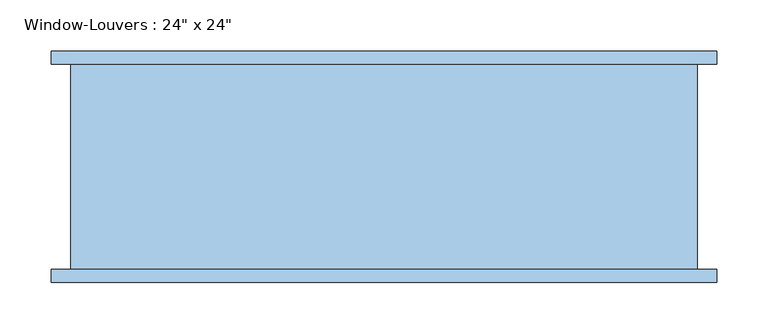
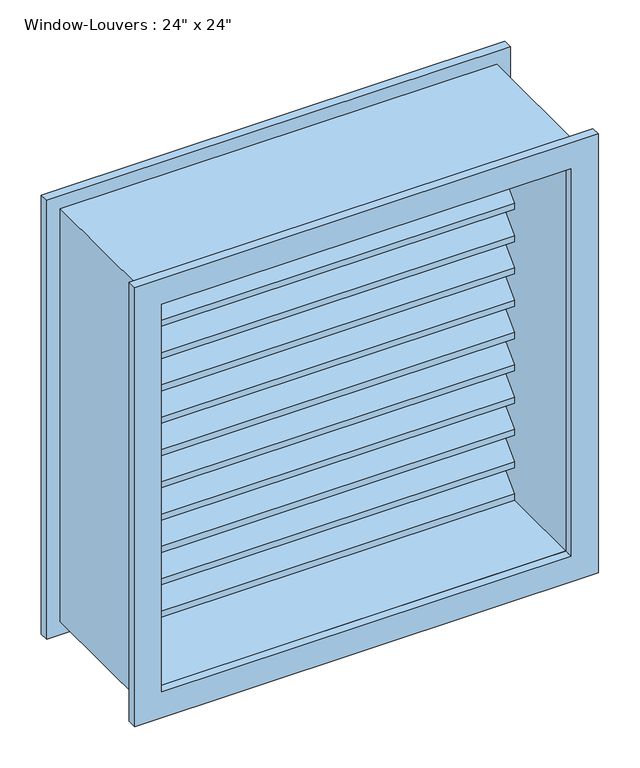
"""IFC4 building model written with IfcOpenShell, lengths in millimetres: window geometry."""

from ifc_helpers import new_model, si_unit, frame, origin, place, context, project, spatial, polyline, outline, extrude, source, transform, mapped, element, save


def window_35a91c22(model_context):
    return source(origin(), model_context, "Body", "SweptSolid", [
        extrude(outline(polyline([(93.65, 1419.1754778), (93.65, 1410.1952217), (55.55, 1448.2952217), (17.45, 1410.1952217), (17.45, 1419.1754778), (55.55, 1457.2754778), (93.65, 1419.1754778)])), frame((-285.75, 0.0, 0.0), z_axis=(1.0, 0.0, 0.0), x_axis=(0.0, 1.0, 0.0)), (0.0, 0.0, 1.0), 571.5),
        extrude(outline(polyline([(93.65, 1371.5009557), (93.65, 1362.5206995), (55.55, 1400.6206995), (17.45, 1362.5206995), (17.45, 1371.5009557), (55.55, 1409.6009557), (93.65, 1371.5009557)])), frame((-285.75, 0.0, 0.0), z_axis=(1.0, 0.0, 0.0), x_axis=(0.0, 1.0, 0.0)), (0.0, 0.0, 1.0), 571.5),
        extrude(outline(polyline([(93.65, 1323.8264335), (93.65, 1314.8461774), (55.55, 1352.9461774), (17.45, 1314.8461774), (17.45, 1323.8264335), (55.55, 1361.9264335), (93.65, 1323.8264335)])), frame((-285.75, 0.0, 0.0), z_axis=(1.0, 0.0, 0.0), x_axis=(0.0, 1.0, 0.0)), (0.0, 0.0, 1.0), 571.5),
        extrude(outline(polyline([(93.65, 1276.1519113), (93.65, 1267.1716552), (55.55, 1305.2716552), (17.45, 1267.1716552), (17.45, 1276.1519113), (55.55, 1314.2519113), (93.65, 1276.1519113)])), frame((-285.75, 0.0, 0.0), z_axis=(1.0, 0.0, 0.0), x_axis=(0.0, 1.0, 0.0)), (0.0, 0.0, 1.0), 571.5),
        extrude(outline(polyline([(93.65, 1228.4773891), (93.65, 1219.497133), (55.55, 1257.597133), (17.45, 1219.497133), (17.45, 1228.4773891), (55.55, 1266.5773891), (93.65, 1228.4773891)])), frame((-285.75, 0.0, 0.0), z_axis=(1.0, 0.0, 0.0), x_axis=(0.0, 1.0, 0.0)), (0.0, 0.0, 1.0), 571.5),
        extrude(outline(polyline([(93.65, 1180.802867), (93.65, 1171.8226109), (55.55, 1209.9226109), (17.45, 1171.8226109), (17.45, 1180.802867), (55.55, 1218.902867), (93.65, 1180.802867)])), frame((-285.75, 0.0, 0.0), z_axis=(1.0, 0.0, 0.0), x_axis=(0.0, 1.0, 0.0)), (0.0, 0.0, 1.0), 571.5),
        extrude(outline(polyline([(93.65, 1133.1283448), (93.65, 1124.1480887), (55.55, 1162.2480887), (17.45, 1124.1480887), (17.45, 1133.1283448), (55.55, 1171.2283448), (93.65, 1133.1283448)])), frame((-285.75, 0.0, 0.0), z_axis=(1.0, 0.0, 0.0), x_axis=(0.0, 1.0, 0.0)), (0.0, 0.0, 1.0), 571.5),
        extrude(outline(polyline([(93.65, 1085.4538226), (93.65, 1076.4735665), (55.55, 1114.5735665), (17.45, 1076.4735665), (17.45, 1085.4538226), (55.55, 1123.5538226), (93.65, 1085.4538226)])), frame((-285.75, 0.0, 0.0), z_axis=(1.0, 0.0, 0.0), x_axis=(0.0, 1.0, 0.0)), (0.0, 0.0, 1.0), 571.5),
        extrude(outline(polyline([(93.65, 1037.7793005), (93.65, 1028.7990443), (55.55, 1066.8990443), (17.45, 1028.7990443), (17.45, 1037.7793005), (55.55, 1075.8793005), (93.65, 1037.7793005)])), frame((-285.75, 0.0, 0.0), z_axis=(1.0, 0.0, 0.0), x_axis=(0.0, 1.0, 0.0)), (0.0, 0.0, 1.0), 571.5),
        extrude(outline(polyline([(93.65, 990.1047783), (93.65, 981.1245222), (55.55, 1019.2245222), (17.45, 981.1245222), (17.45, 990.1047783), (55.55, 1028.2047783), (93.65, 990.1047783)])), frame((-285.75, 0.0, 0.0), z_axis=(1.0, 0.0, 0.0), x_axis=(0.0, 1.0, 0.0)), (0.0, 0.0, 1.0), 571.5),
        extrude(outline(polyline([(93.65, 1466.85), (93.65, 1457.8697439), (55.55, 1495.9697439), (17.45, 1457.8697439), (17.45, 1466.85), (55.55, 1504.95), (93.65, 1466.85)])), frame((-285.75, 0.0, 0.0), z_axis=(1.0, 0.0, 0.0), x_axis=(0.0, 1.0, 0.0)), (0.0, 0.0, 1.0), 571.5),
        extrude(outline(polyline([(93.65, 942.4302561), (93.65, 933.45), (55.55, 971.55), (17.45, 933.45), (17.45, 942.4302561), (55.55, 980.5302561), (93.65, 942.4302561)])), frame((-285.75, 0.0, 0.0), z_axis=(1.0, 0.0, 0.0), x_axis=(0.0, 1.0, 0.0)), (0.0, 0.0, 1.0), 571.5),
        extrude(outline(polyline([(1524.0, 304.8), (1524.0, -304.8), (914.4, -304.8), (914.4, 304.8), (1524.0, 304.8)]), holes=[polyline([(1504.95, 285.75), (933.45, 285.75), (933.45, -285.75), (1504.95, -285.75), (1504.95, 285.75)])]), frame((0.0, -106.35, 0.0), z_axis=(0.0, 1.0, 0.0), x_axis=(0.0, 0.0, 1.0)), (0.0, 0.0, 1.0), 200.0),
        extrude(outline(polyline([(1543.05, 323.85), (1543.05, -323.85), (895.35, -323.85), (895.35, 323.85), (1543.05, 323.85)]), holes=[polyline([(1504.95, 285.75), (933.45, 285.75), (933.45, -285.75), (1504.95, -285.75), (1504.95, 285.75)])]), frame((0.0, -119.05, 0.0), z_axis=(0.0, 1.0, 0.0), x_axis=(0.0, 0.0, 1.0)), (0.0, 0.0, 1.0), 12.7),
        extrude(outline(polyline([(1543.05, -323.85), (895.35, -323.85), (895.35, 323.85), (1543.05, 323.85), (1543.05, -323.85)]), holes=[polyline([(1504.95, -285.75), (1504.95, 285.75), (933.45, 285.75), (933.45, -285.75), (1504.95, -285.75)])]), frame((0.0, 93.65, 0.0), z_axis=(0.0, 1.0, 0.0), x_axis=(0.0, 0.0, 1.0)), (0.0, 0.0, 1.0), 12.7),
    ])


if __name__ == "__main__":
    model = new_model("IFC4")
    model_context = context("Model", 3, world=origin())
    ifc_project = project(units=[si_unit("LENGTHUNIT", "METRE", prefix="MILLI")], contexts=[model_context])
    site = spatial("IfcSite", under=ifc_project)
    building = spatial("IfcBuilding", under=site)
    placement = place(None, origin())
    window_shape = window_35a91c22(model_context)
    element("IfcWindow", 1, ObjectType="Window-Louvers : 24\" x 24\"", at=placement, inside=building, context=model_context, shape_type="MappedRepresentation", body=[
        mapped(window_shape, transform((0.0, 0.0, 0.0), x_axis=(1.0, 0.0, 0.0), y_axis=(0.0, 1.0, 0.0), z_axis=(0.0, 0.0, 1.0))),
    ])
    save(model, "model.ifc")

# Revit data of these elements
# Type "Window-Louvers : 24\" x 24\""
#   Type Mark = "21"
#   Construction Type Id = "GSP4R"
#   Assembly Code = "B20"
#   Analytic Construction = "1/8 in Pilkington single glazing"
#   Visual Light Transmittance = 0.9
#   Thermal Resistance (R) = 1.53941 (h·ft²·°F)/BTU
#   Solar Heat Gain Coefficient = 0.78
#   Max Height = 1' - 11.74264"
#   Height = 2' - 0"
#   Heat Transfer Coefficient (U) = 0.6496 BTU/(h·ft²·°F)
#   Blade Width [instance default] = 1' - 10 1/2"
#   Blade Vertical Thickness = 0' - 0.35355"
#   Blade Thickness = 0' - 0 1/4"
#   Blade Spacing = 0' - 1 1/2"
#   Blade Height = 0' - 1.85355"
#   Blade Depth = 0' - 3"
#   Blade Angle = 45.00°
#   Default Sill Height = 3' - 0"
#   Trim Projection_Exterior = 0' - 0 1/2"
#   Trim Projection_Interior = 0' - 0 1/2"
#   Trim Width_Exterior = 0' - 1 1/2"
#   Trim Width_Interior = 0' - 1 1/2"
#   Width = 2' - 0"
#   Max Blade Count = 12
#   Define Thermal Properties by = 1
#   Blade Count = 12
#   Frame Material = Birch
#   Louver Material = Birch
#   Trim Exterior Material = Birch
#   Trim Interior Material = Birch
#   Wall Closure = (empty or 0)
# Element 1 (IfcWindow, "Window-Louvers : 24\" x 24\"")
#   Materials on its faces: "Birch"
# Materials
#   "Birch": class "Wood", colour RGB 224 178 126, transparency 0, Description = "Betula Alleghaniensis", Cost = 0
